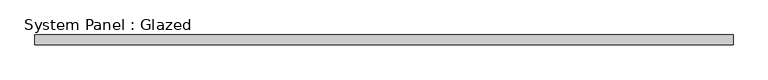
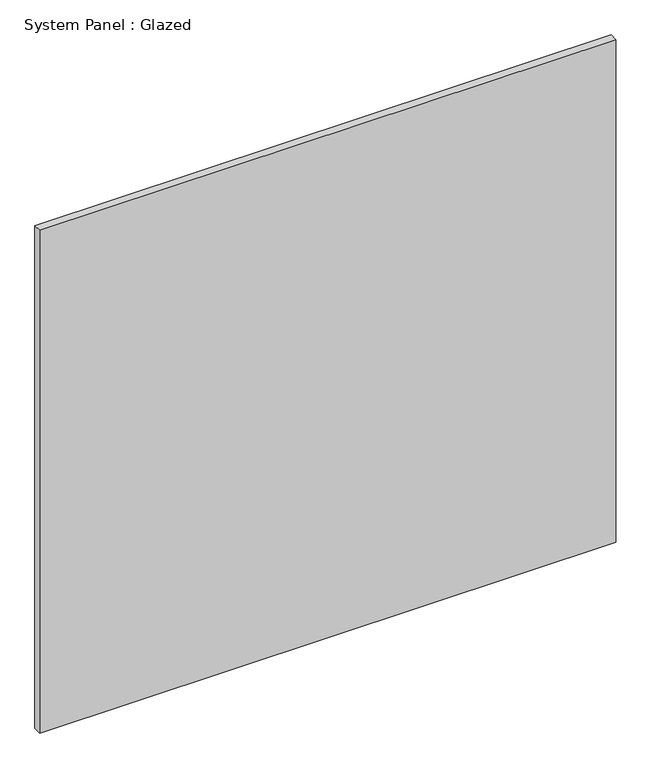
"""IFC4 building model written with IfcOpenShell, lengths in millimetres: plate geometry, System Panel : Glazed."""

from ifc_helpers import new_model, si_unit, origin, origin_with_axes, place, context, project, spatial, polyline, outline, extrude, source, transform, mapped, element, save


def system_panel_glazed_3ebfe8c5(model_context):
    return source(origin(), model_context, "Body", "SweptSolid", [
        extrude(outline(polyline([(912.5143734, 19.05), (-912.5143734, 19.05), (-912.5143734, 44.45), (912.5143734, 44.45), (912.5143734, 19.05)])), origin_with_axes(), (0.0, 0.0, 1.0), 1682.75),
    ])


if __name__ == "__main__":
    model = new_model("IFC4")
    model_context = context("Model", 3, world=origin())
    ifc_project = project(units=[si_unit("LENGTHUNIT", "METRE", prefix="MILLI")], contexts=[model_context])
    site = spatial("IfcSite", under=ifc_project)
    building = spatial("IfcBuilding", under=site)
    placement = place(None, origin())
    system_panel_glazed_shape = system_panel_glazed_3ebfe8c5(model_context)
    element("IfcPlate", 1, ObjectType="System Panel : Glazed", at=placement, inside=building, context=model_context, shape_type="MappedRepresentation", body=[
        mapped(system_panel_glazed_shape, transform((0.0, 0.0, 0.0), x_axis=(1.0, 0.0, 0.0), y_axis=(0.0, 1.0, 0.0), z_axis=(0.0, 0.0, 1.0))),
    ])
    save(model, "model.ifc")

# Revit data of these elements
# Type "System Panel : Glazed"
#   Construction Type Id = "GSP4R"
#   Analytic Construction = "1/8 in Pilkington single glazing"
#   Visual Light Transmittance = 0.9
#   Solar Heat Gain Coefficient = 0.86
#   Heat Transfer Coefficient (U) = 1.18115 BTU/(h·ft²·°F)
# Element 1 (IfcPlate, "System Panel : Glazed")
#   Materials on its faces: "Glass"
# Materials
#   "Glass": class "Glass", colour RGB 0 128 192, transparency 0.75, Description = "Soda Lime Glass", Cost = 0
